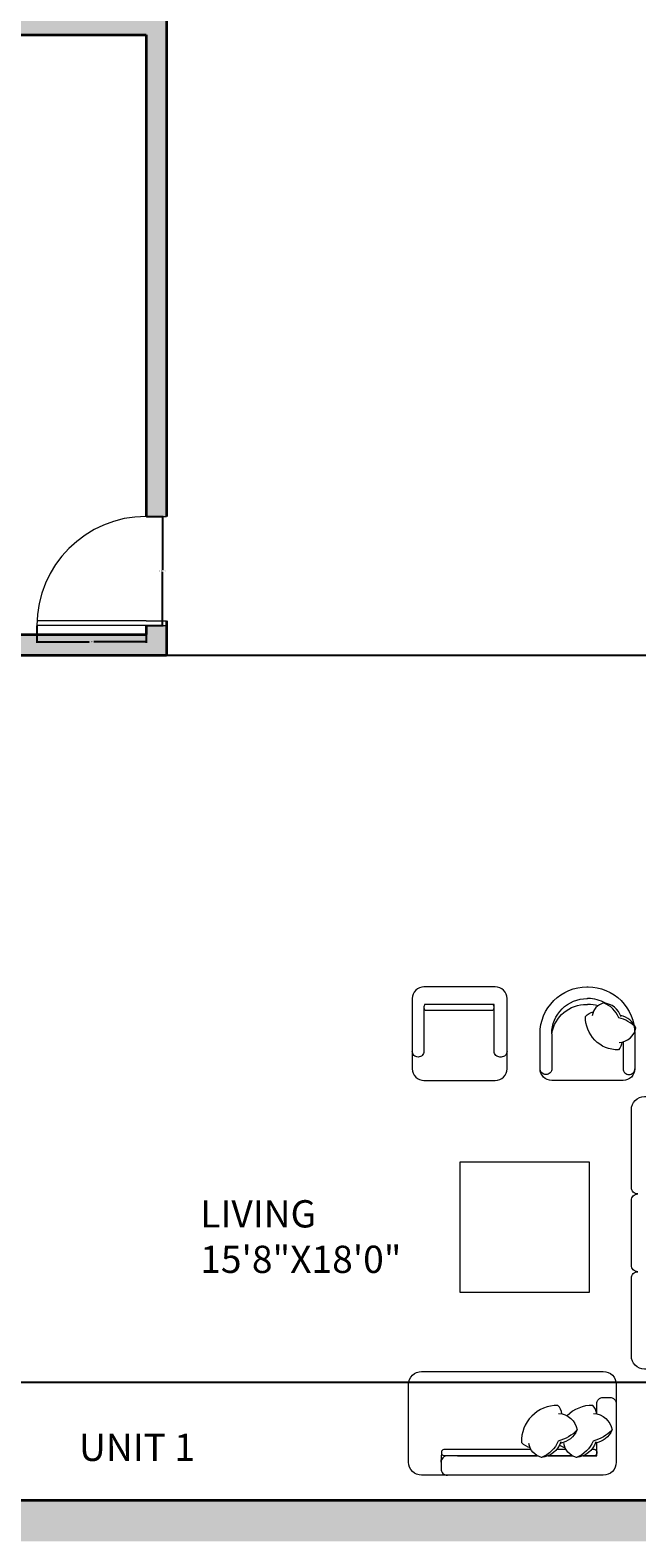
# Model space of a CAD drawing. Units: inches. Extents: x -26 to 13070, y -956 to 6917.
# Tile 7 of 13: x 180 to 314, y -466 to -134. Entities that reach past the tile are written whole.
import ezdxf

# ---------------------------------------------------------------- set-up
doc = ezdxf.new("R2010")
doc.units = ezdxf.units.IN
doc.header["$MEASUREMENT"] = 0
for name, color, linetype, lineweight in [('A-ANNO-DIMS', 2, 'Continuous', 18), ('A-AREA-IDEN', 7, 'Continuous', 18), ('A-DOOR', 3, 'Continuous', 18), ('A-FURN', 8, 'Continuous', 13), ('A-WALL', 7, 'Continuous', 35), ('A-WALL-PATT', 252, 'Continuous', 13)]:
    doc.layers.add(name, color=color, linetype=linetype, lineweight=lineweight)
doc.styles.get("Standard").update_dxf_attribs({"font": 'arial.ttf'})
doc.dimstyles.get("Standard").update_dxf_attribs({"dimtxt": 0.18, "dimasz": 0.18, "dimexe": 0.18, "dimexo": 0.0625, "dimgap": 0.09, "dimtad": 0, "dimtih": 1, "dimtoh": 1, "dimdec": 0, "dimzin": 0, "dimdsep": 46, "dimlunit": 3, "dimtxsty": 'Standard', "dimcen": 0.09, "dimadec": 0, "dimazin": 0, "dimtfac": 1, "dimtdec": 0, "dimtofl": 0, "dimtmove": 0, "dimatfit": 3, "dimfxl": 1, "dimtolj": 1, "dimtzin": 0, "dimarcsym": 0})

# ---------------------------------------------------------------- blocks, each defined once
blk = doc.blocks.new('DAY BED1')
at = {"color": 0}
blk.add_line((0.3, 0.25), (0.225, 0.255), dxfattribs=at)
blk.add_lwpolyline([(-0.3, 0, -0.414214), (-0.4, 0.1), (-0.4, 0.1, 0.317837), (-0.4, 0.1, -0.414214), (-0.4, 0.1), (-0.4, 0.1, 1.186185), (-0.4, 0.1, -0.414214), (-0.4, 0.1), (-0.4, 1.5, -0.414214), (-0.3, 1.6), (0.3, 1.6, -0.414214), (0.4, 1.5), (0.4, 0.1, -0.414214), (0.3, 0)], format="xyb", close=True, dxfattribs=at)
for points in [[(-0.073, 1.45), (-0.15, 1.45, -0.414214), (-0.2, 1.5), (-0.2, 1.55, -0.414214), (-0.15, 1.6)], [(-0.076, 1.425, -0.356772), (0.05, 1.568, -0.249542), (0.154, 1.438, 9.61688)], [(0.05, 1.568, -0.14773), (0.136, 1.422, -0.213343), (0.262, 1.293, -0.178662)], [(-0.073, 1.45, 0.165541), (-0.139, 1.419, 0.200231), (-0.058, 1.221, 0.121523)], [(0.143, 1.442, -0.306663), (0.262, 1.293, -0.30633), (0.154, 1.196, 0.872847)], [(0.25, 1.345), (0.25, 1.45), (0.152, 1.45, -0.414214)], [(0.2, 1.412), (0.2, 1.43, -0.414214), (0.22, 1.45), (0.23, 1.45, -0.414214), (0.25, 1.43)], [(0.25, 1.43), (0.25, 1.345, -0.414214)], [(-0.076, 1.156, -0.356772), (0.05, 1.299, -0.249542), (0.154, 1.169, 9.61688)], [(0.05, 1.299, -0.14773), (0.136, 1.153, -0.213343), (0.262, 1.024, -0.178662)], [(-0.073, 1.181, 0.165541), (-0.139, 1.15, 0.425989), (0.148, 0.869, 0.121523), (0.187, 0.936, -7.115464)], [(0.143, 1.173, -0.306663), (0.262, 1.024, -0.30633), (0.154, 0.926, 0.872847)], [(0.168, 1.163, 0.071865), (0.187, 1.205, -7.115464)], [(0.2, 1.142), (0.2, 1.211, -0.414214)], [(0.25, 1.262), (0.25, 1.075, -0.414214)], [(0.25, 0.992), (0.25, 0.275, -0.414214), (0.23, 0.255), (0.22, 0.255, -0.414214), (0.2, 0.275), (0.2, 0.942, -0.414214)], [(0.25, 0.377), (0.25, 0.3, 0.414214), (0.3, 0.25), (0.35, 0.25, 0.414214), (0.4, 0.3)]]:
    blk.add_lwpolyline(points, format="xyb", dxfattribs=at)
for points in [[(0.25, 1.075), (0.25, 1.262)], [(0.25, 0.377), (0.25, 0.992)]]:
    blk.add_lwpolyline(points, dxfattribs=at)
blk = doc.blocks.new('DOOR-SWING-24')
for p, q in [((24, 1), (0, 1)), ((24, 0), (0, 0))]:
    blk.add_line(p, q)
blk.add_arc((24, 0), 24, 90, 180)
blk = doc.blocks.new('*D14')
at = {"layer": 'A-ANNO-DIMS', "color": 0, "lineweight": -2, "transparency": 16777216}
for p, q in [((205.7, -241.04), (209.42, -241.04)), ((209.24, -241.22), (209.24, -252.86)), ((209.24, -264.86), (209.24, -253.22)), ((205.7, -265.04), (209.42, -265.04))]:
    blk.add_line(p, q, dxfattribs=at)
at = {"layer": 'A-ANNO-DIMS', "color": 0, "transparency": 16777216}
for points in [[(209.21, -241.22), (209.27, -241.22), (209.24, -241.04)], [(209.21, -264.86), (209.27, -264.86), (209.24, -265.04)]]:
    blk.add_solid(points, dxfattribs=at)
at = {"layer": 'Defpoints', "color": 0, "transparency": 16777216}
for p in [(205.64, -241.04), (209.24, -241.04), (205.64, -265.04)]:
    blk.add_point(p, dxfattribs=at)
at = {"layer": 'A-ANNO-DIMS', "color": 0, "transparency": 16777216, "insert": (209.24, -253.04), "char_height": 0.18, "attachment_point": 5}
blk.add_mtext('\\A1;DOOR 24 TYP.', dxfattribs=at)
blk = doc.blocks.new('*D15')
at = {"layer": 'A-ANNO-DIMS', "color": 0, "lineweight": -2, "transparency": 16777216}
for p, q in [((181.64, -265.1), (181.64, -268.82)), ((205.64, -265.1), (205.64, -268.82)), ((181.82, -268.64), (193.11, -268.64)), ((205.46, -268.64), (194.17, -268.64))]:
    blk.add_line(p, q, dxfattribs=at)
at = {"layer": 'A-ANNO-DIMS', "color": 0, "transparency": 16777216}
for points in [[(181.82, -268.61), (181.82, -268.67), (181.64, -268.64)], [(205.46, -268.61), (205.46, -268.67), (205.64, -268.64)]]:
    blk.add_solid(points, dxfattribs=at)
at = {"layer": 'Defpoints', "color": 0, "transparency": 16777216}
for p in [(181.64, -265.04), (205.64, -265.04), (205.64, -268.64)]:
    blk.add_point(p, dxfattribs=at)
at = {"layer": 'A-ANNO-DIMS', "color": 0, "transparency": 16777216, "insert": (193.64, -268.64), "char_height": 0.18, "attachment_point": 5}
blk.add_mtext('\\A1;24 TYP.', dxfattribs=at)
blk = doc.blocks.new('*D41')
at = {"layer": 'A-ANNO-DIMS', "color": 0, "lineweight": -2, "transparency": 16777216}
for p, q in [((214.58, 67.46), (-26.29, 67.46)), ((-26.11, 67.28), (-26.11, -419.86)), ((-26.11, -907.36), (-26.11, -420.22)), ((208.58, -907.54), (-26.29, -907.54))]:
    blk.add_line(p, q, dxfattribs=at)
at = {"layer": 'A-ANNO-DIMS', "color": 0, "transparency": 16777216}
for points in [[(-26.14, 67.28), (-26.08, 67.28), (-26.11, 67.46)], [(-26.14, -907.36), (-26.08, -907.36), (-26.11, -907.54)]]:
    blk.add_solid(points, dxfattribs=at)
at = {"layer": 'Defpoints', "color": 0, "transparency": 16777216}
for p in [(-26.11, 67.46), (214.64, 67.46), (208.64, -907.54)]:
    blk.add_point(p, dxfattribs=at)
at = {"layer": 'A-ANNO-DIMS', "color": 0, "transparency": 16777216, "insert": (-26.11, -420.04), "char_height": 0.18, "attachment_point": 5}
blk.add_mtext('\\A1;975', dxfattribs=at)
blk = doc.blocks.new('*D57')
at = {"layer": 'A-ANNO-DIMS', "color": 0, "lineweight": -2, "transparency": 16777216}
for p, q in [((154.7, -271.54), (596.57, -271.54)), ((596.39, -271.72), (596.39, -351.36)), ((596.39, -431.36), (596.39, -351.72)), ((154.7, -431.54), (596.57, -431.54))]:
    blk.add_line(p, q, dxfattribs=at)
at = {"layer": 'A-ANNO-DIMS', "color": 0, "transparency": 16777216}
for points in [[(596.36, -271.72), (596.42, -271.72), (596.39, -271.54)], [(596.36, -431.36), (596.42, -431.36), (596.39, -431.54)]]:
    blk.add_solid(points, dxfattribs=at)
at = {"layer": 'Defpoints', "color": 0, "transparency": 16777216}
for p in [(154.64, -271.54), (596.39, -271.54), (154.64, -431.54)]:
    blk.add_point(p, dxfattribs=at)
at = {"layer": 'A-ANNO-DIMS', "color": 0, "transparency": 16777216, "insert": (596.39, -351.54), "char_height": 0.18, "attachment_point": 5}
blk.add_mtext('\\A1;160', dxfattribs=at)

msp = doc.modelspace()

# ---------------------------------------------------------------- hatches: boundary and pattern name
at = {"layer": 'A-WALL-PATT'}
h = msp.add_hatch(color=256, dxfattribs=at)
h.dxf.hatch_style = 1
h.paths.add_polyline_path([(223.641, 10.458), (214.641, 10.458), (22.641, 10.458), (22.641, -171.042), (31.641, -171.042), (31.641, -135.042), (205.641, -135.042), (205.641, -241.042), (210.141, -241.042), (210.141, -130.542), (94.641, -130.542), (94.641, -76.542), (85.641, -76.542), (85.641, -126.042), (27.141, -126.042), (27.141, 5.958), (85.641, 5.958), (85.641, -52.542), (94.641, -52.542), (94.641, 1.458), (214.641, 1.458), (214.641, -16.542), (223.641, -16.542), (229.641, -16.542), (229.641, -7.542), (223.641, -7.542)])
h.paths.add_polyline_path([(367.048, 10.458), (346.641, 10.458), (337.641, 10.458), (337.641, -7.542), (331.641, -7.542), (331.641, -16.542), (337.641, -16.542), (342.141, -16.542), (342.141, -128.542), (346.641, -128.542), (346.641, 1.458), (367.048, 1.458)])
h.paths.add_polyline_path([(547.641, 10.458), (403.048, 10.458), (403.048, 1.458), (538.641, 1.458), (538.641, -46.542), (547.641, -46.542)])
h.paths.add_polyline_path([(547.641, -106.542), (538.641, -106.542), (538.641, -154.542), (481.013, -154.542), (481.013, -159.042), (538.641, -159.042), (547.641, -159.042)])
h.paths.add_polyline_path([(457.013, -154.542), (342.141, -154.542), (342.141, -165.042), (346.641, -165.042), (346.641, -159.042), (414.141, -159.042), (414.141, -225.042), (346.641, -225.042), (346.641, -189.042), (342.141, -189.042), (342.141, -234.042), (390.641, -234.042), (390.641, -286.042), (395.141, -286.042), (395.141, -234.042), (456.141, -234.042), (456.141, -312.042), (372.641, -312.042), (372.641, -316.542), (462.641, -316.542), (462.641, -312.042), (460.641, -312.042), (460.641, -234.042), (538.641, -234.042), (547.641, -234.042), (547.641, -195.042), (538.641, -195.042), (538.641, -225.042), (418.641, -225.042), (418.641, -159.042), (457.013, -159.042)])
h.paths.add_polyline_path([(547.641, -270.042), (538.641, -270.042), (538.641, -312.042), (486.641, -312.042), (486.641, -316.542), (538.641, -316.542), (547.641, -316.542)], flags=0)
h.paths.add_polyline_path([(547.641, -456.306), (538.641, -456.306), (538.641, -457.542), (346.641, -457.542), (346.641, -316.542), (346.641, -312.042), (342.141, -312.042), (342.141, -457.542), (145.641, -457.542), (145.641, -466.542), (342.141, -466.542), (342.141, -627.042), (346.641, -627.042), (346.641, -466.542), (538.641, -466.542), (538.641, -514.542), (547.641, -514.542)])
h.paths.add_polyline_path([(466.641, -622.542), (372.641, -622.542), (372.641, -627.042), (388.641, -627.042), (388.641, -721.542), (393.141, -721.542), (393.141, -627.042), (462.141, -627.042), (462.141, -717.042), (466.641, -717.042)])
h.paths.add_polyline_path([(547.641, -574.542), (538.641, -574.542), (538.641, -622.542), (492.641, -622.542), (492.641, -627.042), (538.641, -627.042), (538.641, -654.042), (547.641, -654.042)])
h.paths.add_polyline_path([(547.641, -690.042), (538.641, -690.042), (538.641, -717.042), (466.641, -717.042), (466.641, -721.542), (538.641, -721.542), (538.641, -763.542), (547.641, -763.542)])
h.paths.add_polyline_path([(462.141, -717.042), (419.141, -717.042), (419.141, -721.542), (462.141, -721.542)], flags=0)
h.paths.add_polyline_path([(346.641, -721.542), (352.641, -721.542), (352.641, -717.042), (342.141, -717.042), (342.141, -874.542), (342.141, -907.542), (351.141, -907.542), (351.141, -874.542), (395.949, -874.542), (395.949, -865.542), (351.141, -865.542), (351.141, -841.542), (346.641, -841.542)])
h.paths.add_polyline_path([(547.641, -823.542), (538.641, -823.542), (538.641, -865.542), (431.949, -865.542), (431.949, -874.542), (547.641, -874.542)])
h.paths.add_polyline_path([(172.641, -865.713), (140.641, -865.744), (140.641, -788.744), (182.646, -788.704), (182.641, -784.204), (136.141, -784.249), (136.141, -848.332), (131.641, -848.332), (131.641, -874.542), (172.641, -874.542)])
h.paths.add_polyline_path([(217.641, -816.13), (213.141, -816.13), (213.141, -784.174), (208.641, -784.179), (208.641, -865.679), (208.641, -874.542), (217.641, -874.542)])
h.paths.add_polyline_path([(95.641, -865.788), (31.641, -865.849), (31.641, -832.695), (22.641, -832.695), (22.641, -874.542), (95.641, -874.542)])
h.paths.add_polyline_path([(217.641, -741.17), (31.641, -741.349), (31.641, -708.349), (22.641, -708.349), (22.641, -772.542), (22.641, -796.695), (31.641, -796.695), (31.641, -763.542), (31.641, -745.849), (217.641, -745.67)])
h.paths.add_polyline_path([(31.641, -651.349), (99.65, -651.284), (99.641, -642.284), (31.641, -642.349), (31.641, -639.042), (31.641, -588.349), (125.641, -588.259), (125.641, -651.259), (134.641, -651.25), (134.641, -579.25), (112.641, -579.271), (112.641, -549.042), (112.641, -504.271), (85.633, -504.297), (85.641, -513.297), (103.641, -513.28), (103.641, -549.042), (103.641, -579.28), (31.641, -579.349), (31.641, -549.042), (31.641, -513.349), (49.641, -513.314), (49.633, -504.332), (31.641, -504.349), (22.641, -504.358), (22.641, -684.349), (31.641, -684.349)])
h.paths.add_polyline_path([(31.641, -276.042), (145.641, -276.042), (145.641, -402.042), (145.641, -419.542), (154.641, -419.542), (154.641, -411.042), (154.641, -271.542), (210.141, -271.542), (210.141, -265.042), (205.641, -265.042), (205.641, -267.042), (31.641, -267.042), (31.641, -231.042), (22.641, -231.042), (22.641, -426.852), (31.641, -426.852), (31.641, -411.042), (31.641, -402.042)])

# ---------------------------------------------------------------- linework, layer by layer
at = {"layer": 'A-DOOR'}
for p, q in [((205.641, -241.042), (210.141, -241.042)), ((205.641, -264.042), (210.141, -264.042)), ((205.641, -265.042), (210.141, -265.042))]:
    msp.add_line(p, q, dxfattribs=at)
at = {"layer": 'A-FURN', "ltscale": 0.03}
for points in [[(266.768, -344.552), (266.768, -344.552, 0.4142136), (264.195, -347.125), (264.195, -362.564, 0.4142136), (266.768, -365.138), (266.768, -365.138), (282.465, -365.138, 0.4142136), (285.038, -362.564), (285.038, -347.125, 0.4142136), (282.465, -344.552)], [(315.252, -428.63, -0.4142136), (312.398, -425.776), (312.398, -408.652, -0.4142136), (313.825, -407.225, -0.4142136), (312.398, -405.798), (312.398, -391.528, -0.4142136), (313.825, -390.101, -0.4142136), (312.398, -388.674), (312.398, -371.551, -0.4142136), (315.252, -368.697), (332.376, -368.697, -0.4142136), (335.23, -371.551), (335.23, -425.776, -0.4142136), (332.376, -428.63)]]:
    msp.add_lwpolyline(points, format="xyb", close=True, dxfattribs=at)
msp.add_lwpolyline([(302.734, -365.138), (294.886, -365.138, -0.4142136), (292.313, -362.564), (292.313, -354.845, -0.4142136), (302.606, -344.552), (302.734, -344.552), (302.863, -344.552, -0.4142136), (313.156, -354.845), (313.156, -362.564, -0.4142136), (310.583, -365.138), (302.734, -365.138)], format="xyb", dxfattribs=at)
at = {"layer": 'A-FURN'}
for points in [[(294.886, -354.845, -0.4142136), (302.606, -347.125), (302.734, -347.125)], [(306.695, -348.143, 0.1305915), (302.863, -347.125), (302.734, -347.125)], [(310.125, -351.158, 0.3066635), (306.288, -348.092, 0.30633), (303.781, -350.892, -0.8728472)], [(313.366, -353.546, 0.1477299), (309.606, -351.335, 0.2133428), (306.288, -348.092, 0.1786618)], [(266.768, -349.183), (266.768, -358.704, -0.4142136), (265.482, -359.991), (265.482, -359.991, -0.4142136), (264.195, -358.704)], [(277.361, -348.412), (267.283, -348.412, 0.4142136), (266.768, -348.926), (266.768, -349.183, 0.4142136), (267.283, -349.698), (276.065, -349.698, 0.4142136)], [(276.065, -349.698), (281.693, -349.698, 0.4142136), (282.208, -349.183), (282.208, -348.926, 0.4142136), (281.693, -348.412)], [(281.693, -348.412), (277.361, -348.412, 0.4142136)], [(294.886, -354.845, -0.3727189), (302.606, -348.412), (302.734, -348.412)], [(310.328, -356.71, -0.1655406), (309.532, -358.41, -0.4259892), (302.306, -351.04, -0.1215233), (304.022, -350.024, 7.1154643)], [(305.057, -348.689, 0.0723842), (302.863, -348.412), (302.734, -348.412)], [(309.68, -356.789, 0.3567724), (313.366, -353.546, 0.2495421), (310.026, -350.873, -9.6168803)], [(294.886, -354.844), (294.886, -362.564, -0.4142136), (293.599, -363.851), (293.599, -363.851, -0.4142136), (292.313, -362.564)], [(285.038, -358.704, -0.4142136), (283.752, -359.991), (283.494, -359.991, -0.4142136), (282.208, -358.704), (282.208, -356.711)], [(310.583, -356.649), (310.583, -362.564, 0.4142136), (311.869, -363.851), (311.869, -363.851, 0.4142136), (313.156, -362.564)]]:
    msp.add_lwpolyline(points, format="xyb", dxfattribs=at)
for points in [[(277.361, -348.412), (266.897, -348.412)], [(282.208, -356.711), (282.208, -348.412), (277.361, -348.412)]]:
    msp.add_lwpolyline(points, dxfattribs=at)
at = {"layer": 'A-FURN', "ltscale": 0.03}
msp.add_lwpolyline([(274.623, -383.148), (274.623, -411.687), (303.162, -411.687), (303.162, -383.148)], close=True, dxfattribs=at)
at = {"layer": 'A-WALL'}
for p, q in [((210.141, -130.542), (210.141, -241.042)), ((31.641, -135.042), (205.641, -135.042)), ((205.641, -135.042), (205.641, -241.042)), ((205.641, -265.042), (205.641, -267.042)), ((210.141, -264.042), (210.141, -271.542)), ((31.641, -267.042), (205.641, -267.042)), ((154.641, -271.542), (210.141, -271.542)), ((342.141, -457.542), (145.641, -457.542))]:
    msp.add_line(p, q, dxfattribs=at)

# ---------------------------------------------------------------- block references
at = {"layer": 'A-DOOR'}
msp.add_blockref('DOOR-SWING-24', (181.641, -265.042), dxfattribs=at)
at = {"layer": 'A-FURN', "ltscale": 0.03, "xscale": 28.53951744329711, "yscale": 28.53951744329711, "zscale": 28.53951744329711, "rotation": 270}
msp.add_blockref('DAY BED1', (263.399, -440.586), dxfattribs=at)

# ---------------------------------------------------------------- texts
at = {"layer": 'A-AREA-IDEN', "char_height": 6, "attachment_point": 1}
for s, insert in [('LIVING\\P15\'8"X18\'0"', (217.554, -391.486)), ('UNIT 1', (190.889, -442.86))]:
    msp.add_mtext(s, dxfattribs=dict(at, insert=insert))

# ---------------------------------------------------------------- dimensions: what is measured, and where the dimension line sits
at = {"layer": 'A-ANNO-DIMS'}
for base, p1, p2, picture, middle in [((-26.11, 67.458), (208.641, -907.542), (214.641, 67.458), '*D41', (-26.11, -420.042)), ((596.392, -271.542), (154.641, -431.542), (154.641, -271.542), '*D57', (596.392, -351.542))]:
    dim = msp.add_linear_dim(base=base, p1=p1, p2=p2, angle=90, dimstyle='Standard', override={"dimdec": 0, "dimlfac": 1, "dimrnd": 0, "dimzin": 0, "dimdsep": 46, "dimlunit": 2}, dxfattribs=at)
    dim.commit()
    dim.dimension.update_dxf_attribs({"geometry": picture, "text_midpoint": middle})
dim = msp.add_linear_dim(base=(209.241, -241.042), p1=(205.641, -265.042), p2=(205.641, -241.042), angle=90, text='DOOR <> TYP.', dimstyle='Standard', override={"dimdec": 0, "dimlfac": 1, "dimrnd": 0, "dimzin": 0, "dimdsep": 46, "dimlunit": 2}, dxfattribs=at)
dim.commit()
dim.dimension.update_dxf_attribs({"geometry": '*D14', "text_midpoint": (209.241, -253.042)})
dim = msp.add_linear_dim(base=(205.641, -268.642), p1=(181.641, -265.042), p2=(205.641, -265.042), text='<> TYP.', dimstyle='Standard', override={"dimdec": 0, "dimlfac": 1, "dimrnd": 0, "dimzin": 0, "dimdsep": 46, "dimlunit": 2}, dxfattribs=at)
dim.commit()
dim.dimension.update_dxf_attribs({"geometry": '*D15', "text_midpoint": (193.641, -268.642)})

doc.saveas('drawing.dxf')
